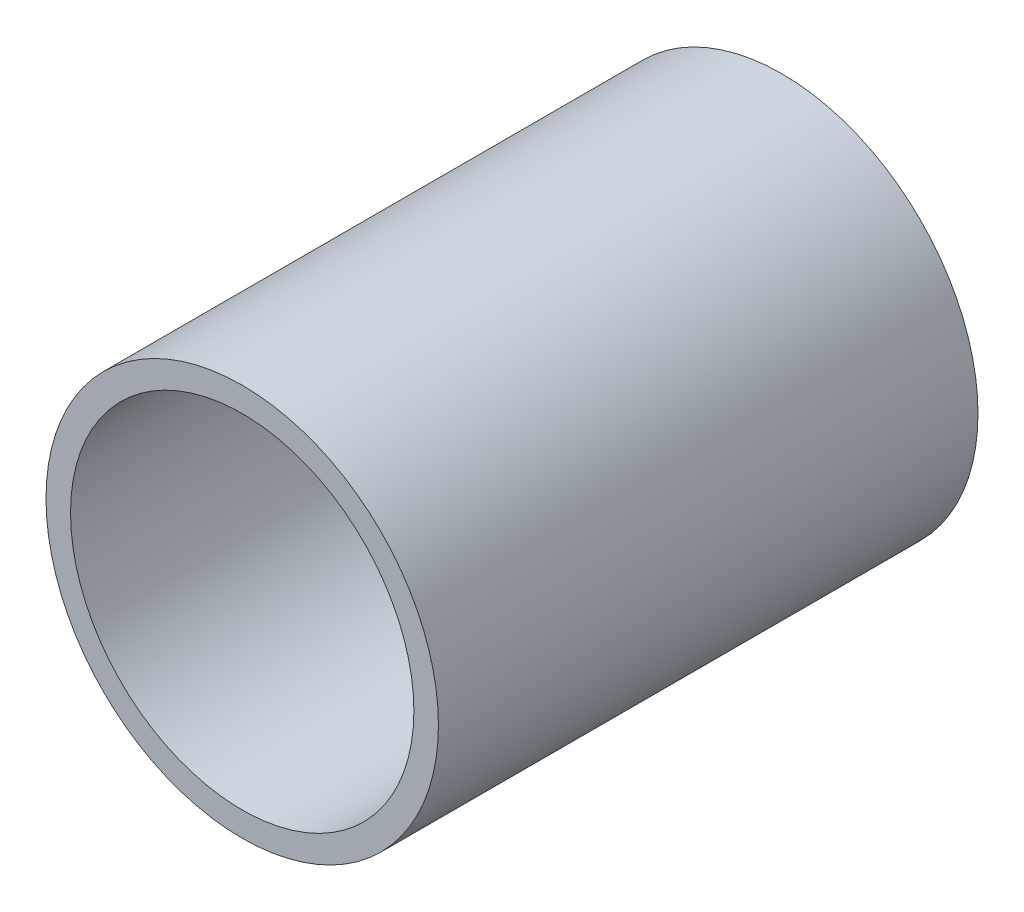
ISO-10303-21;
HEADER;
FILE_DESCRIPTION(('STEP AP214'),'2;1');
FILE_NAME('part.step','',(''),(''),'','','');
FILE_SCHEMA(('AUTOMOTIVE_DESIGN { 1 0 10303 214 1 1 1 1 }'));
ENDSEC;
DATA;
#1=APPLICATION_CONTEXT('core data for automotive mechanical design processes');
#2=APPLICATION_PROTOCOL_DEFINITION('international standard','automotive_design',2000,#1);
#3=PRODUCT_CONTEXT('',#1,'mechanical');
#4=PRODUCT('Part','Part','',(#3));
#5=PRODUCT_RELATED_PRODUCT_CATEGORY('part','',(#4));
#6=PRODUCT_DEFINITION_FORMATION('','',#4);
#7=PRODUCT_DEFINITION_CONTEXT('part definition',#1,'design');
#8=PRODUCT_DEFINITION('design','',#6,#7);
#9=PRODUCT_DEFINITION_SHAPE('','',#8);
#10=(LENGTH_UNIT() NAMED_UNIT(*) SI_UNIT(.MILLI.,.METRE.));
#11=(NAMED_UNIT(*) PLANE_ANGLE_UNIT() SI_UNIT($,.RADIAN.));
#12=(NAMED_UNIT(*) SI_UNIT($,.STERADIAN.) SOLID_ANGLE_UNIT());
#13=UNCERTAINTY_MEASURE_WITH_UNIT(LENGTH_MEASURE(1.E-05),#10,'distance_accuracy_value','');
#14=(GEOMETRIC_REPRESENTATION_CONTEXT(3) GLOBAL_UNCERTAINTY_ASSIGNED_CONTEXT((#13)) GLOBAL_UNIT_ASSIGNED_CONTEXT((#10,
#11,#12)) REPRESENTATION_CONTEXT('',''));
#15=CARTESIAN_POINT('',(0.,0.,0.));
#16=DIRECTION('',(0.,0.,1.));
#17=DIRECTION('',(1.,0.,0.));
#18=AXIS2_PLACEMENT_3D('',#15,#16,#17);
#19=CARTESIAN_POINT('',(0.,0.,110.));
#20=DIRECTION('',(0.,0.,1.));
#21=DIRECTION('',(1.,0.,0.));
#22=AXIS2_PLACEMENT_3D('',#19,#20,#21);
#23=PLANE('',#22);
#24=CARTESIAN_POINT('',(0.,0.,110.));
#25=DIRECTION('',(0.,0.,1.));
#26=DIRECTION('',(1.,0.,0.));
#27=AXIS2_PLACEMENT_3D('',#24,#25,#26);
#28=CIRCLE('',#27,40.);
#29=CARTESIAN_POINT('',(40.,0.,110.));
#30=VERTEX_POINT('',#29);
#31=EDGE_CURVE('E10',#30,#30,#28,.T.);
#32=ORIENTED_EDGE('',*,*,#31,.T.);
#33=EDGE_LOOP('',(#32));
#34=FACE_BOUND('',#33,.T.);
#35=CARTESIAN_POINT('',(0.,0.,110.));
#36=DIRECTION('',(0.,0.,1.));
#37=DIRECTION('',(1.,0.,0.));
#38=AXIS2_PLACEMENT_3D('',#35,#36,#37);
#39=CIRCLE('',#38,35.);
#40=CARTESIAN_POINT('',(35.,0.,110.));
#41=VERTEX_POINT('',#40);
#42=EDGE_CURVE('E49',#41,#41,#39,.T.);
#43=ORIENTED_EDGE('',*,*,#42,.F.);
#44=EDGE_LOOP('',(#43));
#45=FACE_BOUND('',#44,.T.);
#46=ADVANCED_FACE('F39',(#34,#45),#23,.T.);
#47=CARTESIAN_POINT('',(0.,0.,0.));
#48=DIRECTION('',(0.,0.,1.));
#49=DIRECTION('',(1.,0.,0.));
#50=AXIS2_PLACEMENT_3D('',#47,#48,#49);
#51=PLANE('',#50);
#52=CARTESIAN_POINT('',(0.,0.,0.));
#53=DIRECTION('',(0.,0.,1.));
#54=DIRECTION('',(1.,0.,0.));
#55=AXIS2_PLACEMENT_3D('',#52,#53,#54);
#56=CIRCLE('',#55,40.);
#57=CARTESIAN_POINT('',(40.,0.,0.));
#58=VERTEX_POINT('',#57);
#59=EDGE_CURVE('E43',#58,#58,#56,.T.);
#60=ORIENTED_EDGE('',*,*,#59,.F.);
#61=EDGE_LOOP('',(#60));
#62=FACE_BOUND('',#61,.T.);
#63=CARTESIAN_POINT('',(0.,0.,0.));
#64=DIRECTION('',(0.,0.,1.));
#65=DIRECTION('',(1.,0.,0.));
#66=AXIS2_PLACEMENT_3D('',#63,#64,#65);
#67=CIRCLE('',#66,35.);
#68=CARTESIAN_POINT('',(35.,0.,0.));
#69=VERTEX_POINT('',#68);
#70=EDGE_CURVE('E55',#69,#69,#67,.T.);
#71=ORIENTED_EDGE('',*,*,#70,.T.);
#72=EDGE_LOOP('',(#71));
#73=FACE_BOUND('',#72,.T.);
#74=ADVANCED_FACE('F65',(#62,#73),#51,.F.);
#75=CARTESIAN_POINT('',(0.,0.,110.));
#76=DIRECTION('',(0.,0.,-1.));
#77=DIRECTION('',(-1.,0.,0.));
#78=AXIS2_PLACEMENT_3D('',#75,#76,#77);
#79=CYLINDRICAL_SURFACE('',#78,40.);
#80=ORIENTED_EDGE('',*,*,#31,.F.);
#81=EDGE_LOOP('',(#80));
#82=FACE_BOUND('',#81,.T.);
#83=ORIENTED_EDGE('',*,*,#59,.T.);
#84=EDGE_LOOP('',(#83));
#85=FACE_BOUND('',#84,.T.);
#86=ADVANCED_FACE('F41',(#82,#85),#79,.T.);
#87=CARTESIAN_POINT('',(0.,0.,110.));
#88=DIRECTION('',(0.,0.,-1.));
#89=DIRECTION('',(-1.,0.,0.));
#90=AXIS2_PLACEMENT_3D('',#87,#88,#89);
#91=CYLINDRICAL_SURFACE('',#90,35.);
#92=ORIENTED_EDGE('',*,*,#42,.T.);
#93=EDGE_LOOP('',(#92));
#94=FACE_BOUND('',#93,.T.);
#95=ORIENTED_EDGE('',*,*,#70,.F.);
#96=EDGE_LOOP('',(#95));
#97=FACE_BOUND('',#96,.T.);
#98=ADVANCED_FACE('F59',(#94,#97),#91,.F.);
#99=CLOSED_SHELL('',(#46,#74,#86,#98));
#100=MANIFOLD_SOLID_BREP('B2',#99);
#101=ADVANCED_BREP_SHAPE_REPRESENTATION('',(#18,#100),#14);
#102=SHAPE_DEFINITION_REPRESENTATION(#9,#101);
ENDSEC;
END-ISO-10303-21;
